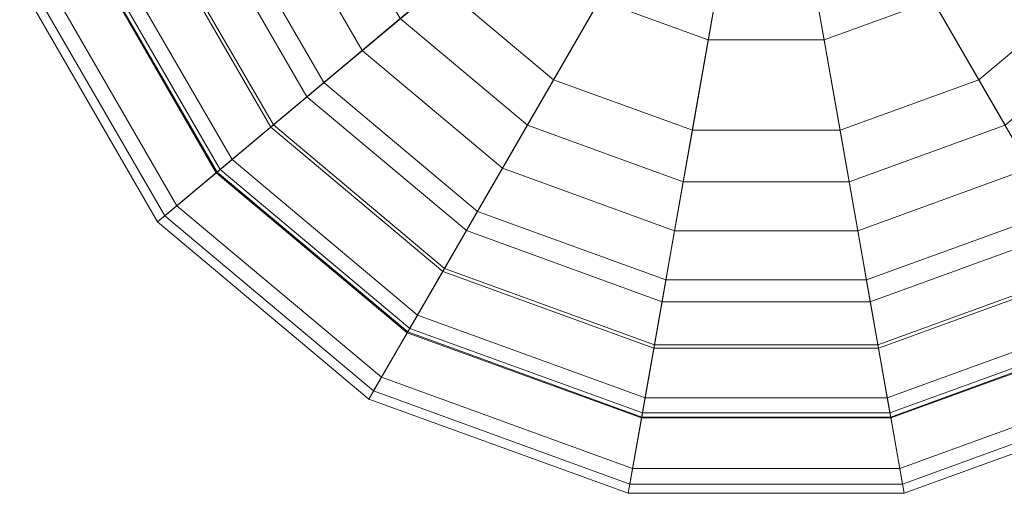
# Model space of a CAD drawing. Units: inches. Extents: x 375 to 1122, y 27 to 1069.
# Tile 119 of 155: x 717.991 to 719.669, y 889.781 to 890.59. Entities that reach past the tile are written whole.
import ezdxf

# ---------------------------------------------------------------- set-up
doc = ezdxf.new("R2010")
doc.units = ezdxf.units.IN
doc.layers.add('Furniture', color=30, linetype='Continuous', lineweight=18)

# ---------------------------------------------------------------- blocks, each defined once
blk = doc.blocks.new('A$C403C54AD')
for points in [[(1.202018, 0.883824, -0.031825), (1.180252, 0.857884, -0.028747), (1.180252, 0.857884, -0.028747), (1.191834, 0.889704, -0.031825)], [(1.209578, 0.874815, -0.031825), (1.180252, 0.857884, -0.028747), (1.180252, 0.857884, -0.028747), (1.202018, 0.883824, -0.031825)], [(1.192562, 0.864991, -0.02532), (1.206749, 0.873182, -0.028594), (1.199919, 0.881322, -0.028594), (1.189389, 0.868773, -0.02532)], [(1.195951, 0.866948, 0.063639), (1.201568, 0.87019, 0.073031), (1.196073, 0.876739, 0.073031), (1.191904, 0.87177, 0.063639)], [(1.2136, 0.863764, -0.031825), (1.180252, 0.857884, -0.028747), (1.180252, 0.857884, -0.028747), (1.209578, 0.874815, -0.031825)], [(1.210384, 0.863197, -0.028594), (1.2136, 0.863764, -0.031825), (1.209578, 0.874815, -0.031825), (1.206749, 0.873182, -0.028594)], [(1.212542, 0.863578, 0.089693), (1.207259, 0.862646, 0.071684), (1.204002, 0.871596, 0.071684), (1.208648, 0.874278, 0.089693)], [(1.210344, 0.86319, 0.131159), (1.213207, 0.863695, 0.117935), (1.209232, 0.874616, 0.117935), (1.206714, 0.873162, 0.131159)], [(1.213207, 0.863695, 0.117935), (1.212542, 0.863578, 0.089693), (1.208648, 0.874278, 0.089693), (1.209232, 0.874616, 0.117935)], [(1.197882, 0.868063, 0.061451), (1.189015, 0.862943, 0.054084), (1.186756, 0.865635, 0.054084), (1.193338, 0.873479, 0.061451)], [(1.19425, 0.860352, -0.02532), (1.210384, 0.863197, -0.028594), (1.206749, 0.873182, -0.028594), (1.192562, 0.864991, -0.02532)], [(1.205423, 0.862322, 0.140564), (1.210344, 0.86319, 0.131159), (1.206714, 0.873162, 0.131159), (1.202387, 0.870664, 0.140564)], [(1.210169, 0.863159, 0.117718), (1.207402, 0.862671, 0.130354), (1.204128, 0.871669, 0.130354), (1.206561, 0.873073, 0.117718)], [(1.209521, 0.863045, 0.090178), (1.210169, 0.863159, 0.117718), (1.206561, 0.873073, 0.117718), (1.205991, 0.872744, 0.090178)], [(1.204491, 0.862158, 0.073031), (1.209521, 0.863045, 0.090178), (1.205991, 0.872744, 0.090178), (1.201568, 0.87019, 0.073031)], [(1.187963, 0.862336, 0.057003), (1.195951, 0.866948, 0.063639), (1.191904, 0.87177, 0.063639), (1.185975, 0.864705, 0.057003)], [(1.207259, 0.862646, 0.071684), (1.2003, 0.861419, 0.061451), (1.197882, 0.868063, 0.061451), (1.204002, 0.871596, 0.071684)], [(1.207402, 0.862671, 0.130354), (1.202392, 0.861788, 0.140564), (1.199721, 0.869125, 0.140564), (1.204128, 0.871669, 0.130354)], [(1.202392, 0.861788, 0.140564), (1.205423, 0.862322, 0.140564), (1.202387, 0.870664, 0.140564), (1.199721, 0.869125, 0.140564)], [(1.198104, 0.861032, 0.063639), (1.204491, 0.862158, 0.073031), (1.201568, 0.87019, 0.073031), (1.195951, 0.866948, 0.063639)], [(1.2003, 0.861419, 0.061451), (1.190217, 0.859641, 0.054084), (1.189015, 0.862943, 0.054084), (1.197882, 0.868063, 0.061451)], [(1.189021, 0.85943, 0.057003), (1.198104, 0.861032, 0.063639), (1.195951, 0.866948, 0.063639), (1.187963, 0.862336, 0.057003)], [(1.192234, 0.859997, -0.022455), (1.19425, 0.860352, -0.02532), (1.192562, 0.864991, -0.02532), (1.190789, 0.863967, -0.022455)], [(1.2136, 0.852004, -0.031825), (1.180252, 0.857884, -0.028747), (1.180252, 0.857884, -0.028747), (1.2136, 0.863764, -0.031825)], [(1.210384, 0.852571, -0.028594), (1.2136, 0.852004, -0.031825), (1.2136, 0.863764, -0.031825), (1.210384, 0.863197, -0.028594)], [(1.212542, 0.85219, 0.089693), (1.207259, 0.853122, 0.071684), (1.207259, 0.862646, 0.071684), (1.212542, 0.863578, 0.089693)], [(1.210344, 0.852578, 0.131159), (1.213207, 0.852073, 0.117935), (1.213207, 0.863695, 0.117935), (1.210344, 0.86319, 0.131159)], [(1.213207, 0.852073, 0.117935), (1.212542, 0.85219, 0.089693), (1.212542, 0.863578, 0.089693), (1.213207, 0.863695, 0.117935)], [(1.19425, 0.855416, -0.02532), (1.210384, 0.852571, -0.028594), (1.210384, 0.863197, -0.028594), (1.19425, 0.860352, -0.02532)], [(1.204491, 0.85361, 0.073031), (1.209521, 0.852723, 0.090178), (1.209521, 0.863045, 0.090178), (1.204491, 0.862158, 0.073031)], [(1.205423, 0.853446, 0.140564), (1.210344, 0.852578, 0.131159), (1.210344, 0.86319, 0.131159), (1.205423, 0.862322, 0.140564)], [(1.210169, 0.852609, 0.117718), (1.207402, 0.853097, 0.130354), (1.207402, 0.862671, 0.130354), (1.210169, 0.863159, 0.117718)], [(1.209521, 0.852723, 0.090178), (1.210169, 0.852609, 0.117718), (1.210169, 0.863159, 0.117718), (1.209521, 0.863045, 0.090178)], [(1.207259, 0.853122, 0.071684), (1.2003, 0.854349, 0.061451), (1.2003, 0.861419, 0.061451), (1.207259, 0.862646, 0.071684)], [(1.207402, 0.853097, 0.130354), (1.202392, 0.85398, 0.140564), (1.202392, 0.861788, 0.140564), (1.207402, 0.862671, 0.130354)], [(1.198104, 0.854736, 0.063639), (1.204491, 0.85361, 0.073031), (1.204491, 0.862158, 0.073031), (1.198104, 0.861032, 0.063639)], [(1.202392, 0.85398, 0.140564), (1.205423, 0.853446, 0.140564), (1.205423, 0.862322, 0.140564), (1.202392, 0.861788, 0.140564)], [(1.2003, 0.854349, 0.061451), (1.190217, 0.856127, 0.054084), (1.190217, 0.859641, 0.054084), (1.2003, 0.861419, 0.061451)], [(1.189021, 0.856338, 0.057003), (1.198104, 0.854736, 0.063639), (1.198104, 0.861032, 0.063639), (1.189021, 0.85943, 0.057003)], [(1.192234, 0.855771, -0.022455), (1.19425, 0.855416, -0.02532), (1.19425, 0.860352, -0.02532), (1.192234, 0.859997, -0.022455)], [(1.209578, 0.840953, -0.031825), (1.180252, 0.857884, -0.028747), (1.180252, 0.857884, -0.028747), (1.2136, 0.852004, -0.031825)], [(1.202018, 0.831944, -0.031825), (1.180252, 0.857884, -0.028747), (1.180252, 0.857884, -0.028747), (1.209578, 0.840953, -0.031825)], [(1.191834, 0.826064, -0.031825), (1.180252, 0.857884, -0.028747), (1.180252, 0.857884, -0.028747), (1.202018, 0.831944, -0.031825)], [(1.187963, 0.853432, 0.057003), (1.195951, 0.84882, 0.063639), (1.198104, 0.854736, 0.063639), (1.189021, 0.856338, 0.057003)], [(1.197882, 0.847705, 0.061451), (1.189015, 0.852825, 0.054084), (1.190217, 0.856127, 0.054084), (1.2003, 0.854349, 0.061451)], [(1.190789, 0.851801, -0.022455), (1.192562, 0.850777, -0.02532), (1.19425, 0.855416, -0.02532), (1.192234, 0.855771, -0.022455)], [(1.192562, 0.850777, -0.02532), (1.206749, 0.842586, -0.028594), (1.210384, 0.852571, -0.028594), (1.19425, 0.855416, -0.02532)], [(1.195951, 0.84882, 0.063639), (1.201568, 0.845577, 0.073031), (1.204491, 0.85361, 0.073031), (1.198104, 0.854736, 0.063639)], [(1.204002, 0.844172, 0.071684), (1.197882, 0.847705, 0.061451), (1.2003, 0.854349, 0.061451), (1.207259, 0.853122, 0.071684)], [(1.199721, 0.846643, 0.140564), (1.202387, 0.845104, 0.140564), (1.205423, 0.853446, 0.140564), (1.202392, 0.85398, 0.140564)], [(1.204128, 0.844099, 0.130354), (1.199721, 0.846643, 0.140564), (1.202392, 0.85398, 0.140564), (1.207402, 0.853097, 0.130354)], [(1.185975, 0.851063, 0.057003), (1.191904, 0.843998, 0.063639), (1.195951, 0.84882, 0.063639), (1.187963, 0.853432, 0.057003)], [(1.201568, 0.845577, 0.073031), (1.205991, 0.843024, 0.090178), (1.209521, 0.852723, 0.090178), (1.204491, 0.85361, 0.073031)], [(1.202387, 0.845104, 0.140564), (1.206714, 0.842606, 0.131159), (1.210344, 0.852578, 0.131159), (1.205423, 0.853446, 0.140564)], [(1.193338, 0.842289, 0.061451), (1.186756, 0.850133, 0.054084), (1.189015, 0.852825, 0.054084), (1.197882, 0.847705, 0.061451)], [(1.208648, 0.84149, 0.089693), (1.204002, 0.844172, 0.071684), (1.207259, 0.853122, 0.071684), (1.212542, 0.85219, 0.089693)], [(1.206561, 0.842695, 0.117718), (1.204128, 0.844099, 0.130354), (1.207402, 0.853097, 0.130354), (1.210169, 0.852609, 0.117718)], [(1.205991, 0.843024, 0.090178), (1.206561, 0.842695, 0.117718), (1.210169, 0.852609, 0.117718), (1.209521, 0.852723, 0.090178)], [(1.206714, 0.842606, 0.131159), (1.209232, 0.841152, 0.117935), (1.213207, 0.852073, 0.117935), (1.210344, 0.852578, 0.131159)], [(1.206749, 0.842586, -0.028594), (1.209578, 0.840953, -0.031825), (1.2136, 0.852004, -0.031825), (1.210384, 0.852571, -0.028594)], [(1.209232, 0.841152, 0.117935), (1.208648, 0.84149, 0.089693), (1.212542, 0.85219, 0.089693), (1.213207, 0.852073, 0.117935)], [(1.189389, 0.846995, -0.02532), (1.199919, 0.834446, -0.028594), (1.206749, 0.842586, -0.028594), (1.192562, 0.850777, -0.02532)], [(1.191904, 0.843998, 0.063639), (1.196073, 0.839029, 0.073031), (1.201568, 0.845577, 0.073031), (1.195951, 0.84882, 0.063639)], [(1.19788, 0.836876, 0.071684), (1.193338, 0.842289, 0.061451), (1.197882, 0.847705, 0.061451), (1.204002, 0.844172, 0.071684)], [(1.185114, 0.844527, -0.02532), (1.190717, 0.829133, -0.028594), (1.199919, 0.834446, -0.028594), (1.189389, 0.846995, -0.02532)], [(1.194703, 0.840662, 0.140564), (1.196681, 0.838304, 0.140564), (1.202387, 0.845104, 0.140564), (1.199721, 0.846643, 0.140564)], [(1.197973, 0.836765, 0.130354), (1.194703, 0.840662, 0.140564), (1.199721, 0.846643, 0.140564), (1.204128, 0.844099, 0.130354)], [(1.196073, 0.839029, 0.073031), (1.199356, 0.835117, 0.090178), (1.205991, 0.843024, 0.090178), (1.201568, 0.845577, 0.073031)], [(1.196681, 0.838304, 0.140564), (1.199893, 0.834477, 0.131159), (1.206714, 0.842606, 0.131159), (1.202387, 0.845104, 0.140564)], [(1.186452, 0.84085, 0.063639), (1.18867, 0.834755, 0.073031), (1.196073, 0.839029, 0.073031), (1.191904, 0.843998, 0.063639)], [(1.201328, 0.832767, 0.089693), (1.19788, 0.836876, 0.071684), (1.204002, 0.844172, 0.071684), (1.208648, 0.84149, 0.089693)], [(1.199779, 0.834612, 0.117718), (1.197973, 0.836765, 0.130354), (1.204128, 0.844099, 0.130354), (1.206561, 0.842695, 0.117718)], [(1.199356, 0.835117, 0.090178), (1.199779, 0.834612, 0.117718), (1.206561, 0.842695, 0.117718), (1.205991, 0.843024, 0.090178)], [(1.199893, 0.834477, 0.131159), (1.201762, 0.83225, 0.117935), (1.209232, 0.841152, 0.117935), (1.206714, 0.842606, 0.131159)], [(1.199919, 0.834446, -0.028594), (1.202018, 0.831944, -0.031825), (1.209578, 0.840953, -0.031825), (1.206749, 0.842586, -0.028594)], [(1.189632, 0.832114, 0.071684), (1.187215, 0.838754, 0.061451), (1.193338, 0.842289, 0.061451), (1.19788, 0.836876, 0.071684)], [(1.201762, 0.83225, 0.117935), (1.201328, 0.832767, 0.089693), (1.208648, 0.84149, 0.089693), (1.209232, 0.841152, 0.117935)], [(1.187941, 0.836759, 0.140564), (1.188994, 0.833866, 0.140564), (1.196681, 0.838304, 0.140564), (1.194703, 0.840662, 0.140564)], [(1.189681, 0.831977, 0.130354), (1.187941, 0.836759, 0.140564), (1.194703, 0.840662, 0.140564), (1.197973, 0.836765, 0.130354)], [(1.18867, 0.834755, 0.073031), (1.190417, 0.829956, 0.090178), (1.199356, 0.835117, 0.090178), (1.196073, 0.839029, 0.073031)], [(1.188994, 0.833866, 0.140564), (1.190703, 0.829171, 0.131159), (1.199893, 0.834477, 0.131159), (1.196681, 0.838304, 0.140564)], [(1.191466, 0.827073, 0.089693), (1.189632, 0.832114, 0.071684), (1.19788, 0.836876, 0.071684), (1.201328, 0.832767, 0.089693)], [(1.190642, 0.829337, 0.117718), (1.189681, 0.831977, 0.130354), (1.197973, 0.836765, 0.130354), (1.199779, 0.834612, 0.117718)], [(1.190417, 0.829956, 0.090178), (1.190642, 0.829337, 0.117718), (1.199779, 0.834612, 0.117718), (1.199356, 0.835117, 0.090178)], [(1.190703, 0.829171, 0.131159), (1.191697, 0.826439, 0.117935), (1.201762, 0.83225, 0.117935), (1.199893, 0.834477, 0.131159)], [(1.190717, 0.829133, -0.028594), (1.191834, 0.826064, -0.031825), (1.202018, 0.831944, -0.031825), (1.199919, 0.834446, -0.028594)], [(1.191697, 0.826439, 0.117935), (1.191466, 0.827073, 0.089693), (1.201328, 0.832767, 0.089693), (1.201762, 0.83225, 0.117935)]]:
    blk.add_3dface(points)

msp = doc.modelspace()

# ---------------------------------------------------------------- block references
at = {"layer": 'Furniture', "xscale": 39.9918517141215, "yscale": 39.9918517141215, "zscale": 39.9918517141215, "rotation": 270}
msp.add_blockref('A$C403C54AD', (684.9549, 938.3156, 0.024), dxfattribs=at)

doc.saveas('drawing.dxf')
